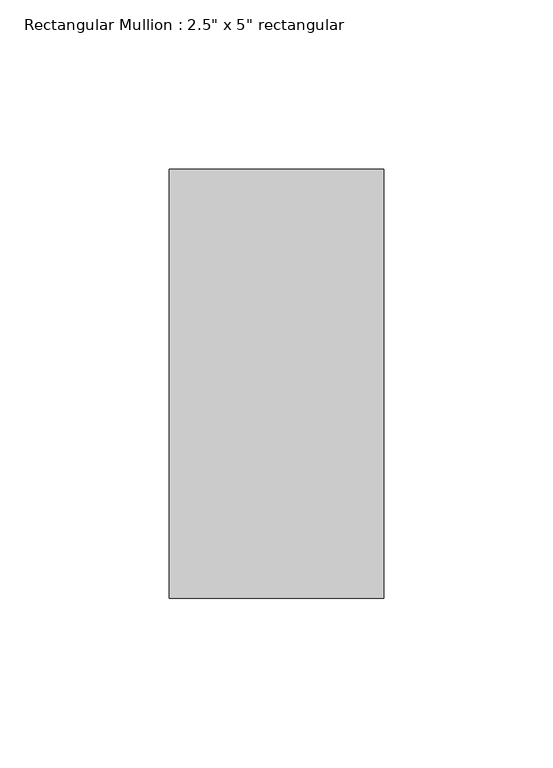
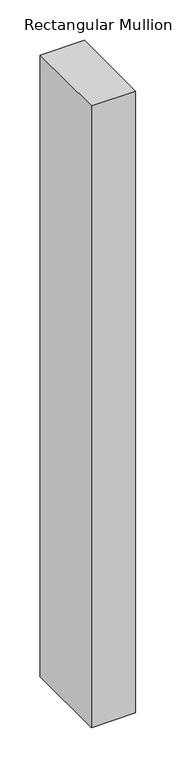
"""IFC4 building model written with IfcOpenShell, lengths in millimetres: member geometry."""

from ifc_helpers import new_model, si_unit, frame, origin, place, context, project, spatial, polyline, outline, extrude, source, transform, mapped, element, save


def member_f2949ae1(model_context):
    return source(origin(), model_context, "Body", "SweptSolid", [
        extrude(outline(polyline([(31.75, 63.5), (31.75, -63.5), (-31.75, -63.5), (-31.75, 63.5), (31.75, 63.5)])), frame((0.0, 0.0, -940.9162788), z_axis=(0.0, 0.0, 1.0), x_axis=(1.0, 0.0, 0.0)), (0.0, 0.0, 1.0), 940.9162788),
    ])


if __name__ == "__main__":
    model = new_model("IFC4")
    model_context = context("Model", 3, world=origin())
    ifc_project = project(units=[si_unit("LENGTHUNIT", "METRE", prefix="MILLI")], contexts=[model_context])
    site = spatial("IfcSite", under=ifc_project)
    building = spatial("IfcBuilding", under=site)
    placement = place(None, origin())
    member_shape = member_f2949ae1(model_context)
    element("IfcMember", 1, ObjectType="Rectangular Mullion : 2.5\" x 5\" rectangular", at=placement, inside=building, context=model_context, shape_type="MappedRepresentation", body=[
        mapped(member_shape, transform((0.0, 0.0, 0.0), x_axis=(1.0, 0.0, 0.0), y_axis=(0.0, 1.0, 0.0), z_axis=(0.0, 0.0, 1.0))),
    ])
    save(model, "model.ifc")

# Revit data of these elements
# Type "Rectangular Mullion : 2.5\" x 5\" rectangular"
#   built-in parameter 1007304 = 0.416667 (stored number, unit not read)
#   built-in parameter 1007301 = 0.104167 (stored number, unit not read)
#   built-in parameter 1007300 = 0.104167 (stored number, unit not read)
# Element 1 (IfcMember, "Rectangular Mullion : 2.5\" x 5\" rectangular")
#   Materials on its faces: "Aluminum"
# Materials
#   "Aluminum": class "Metal", colour RGB 247 247 247, transparency 0, Description = "Aluminum 6061", Cost = 0
